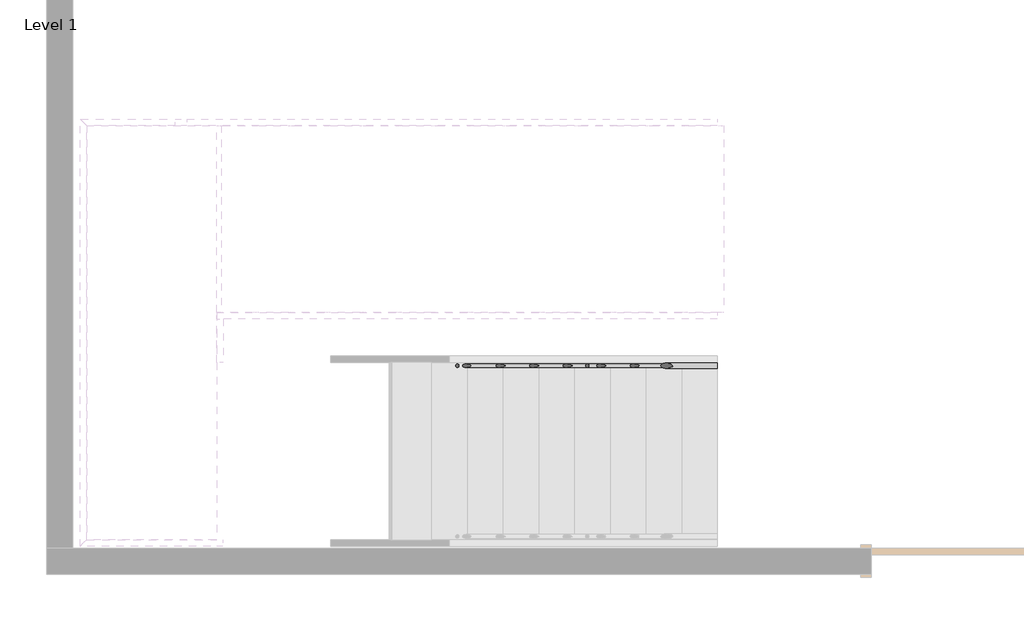
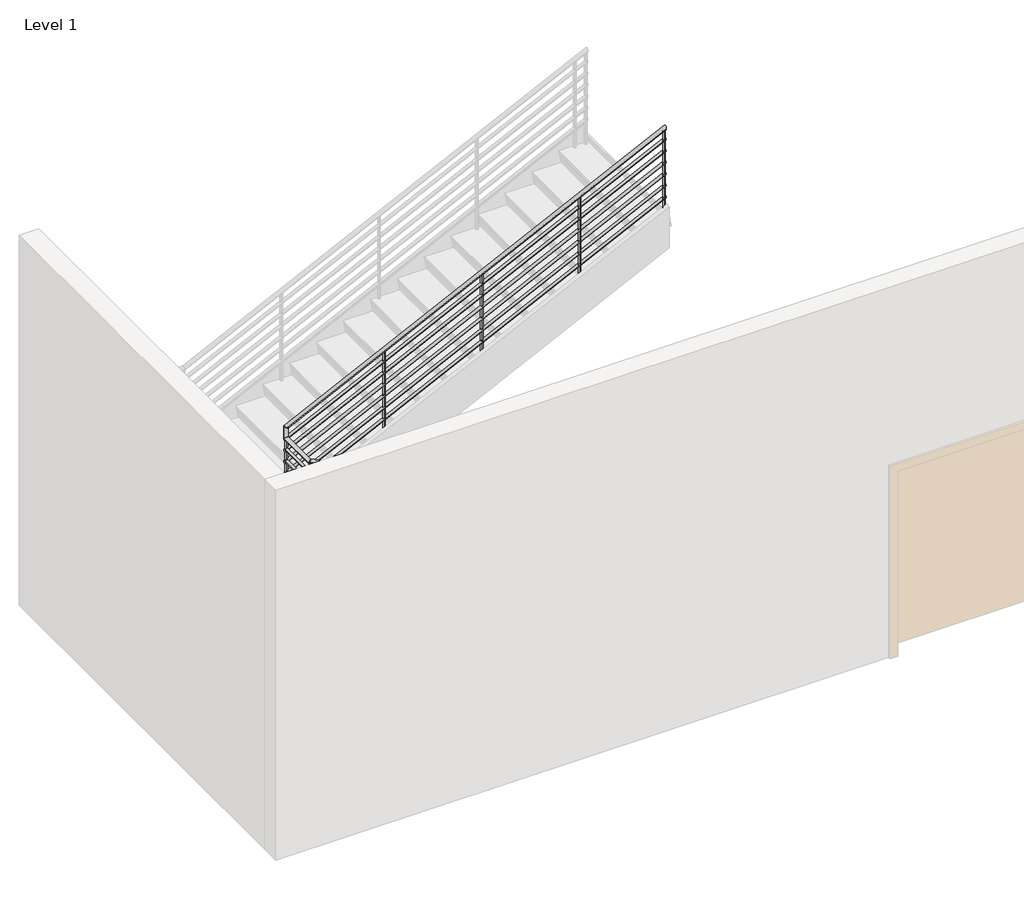
# One storey, part 2 of 4: 1 railing.
"""IFC4 building model written with IfcOpenShell, lengths in millimetres."""

from ifc_helpers import new_model, si_unit, point, frame, frame_2d, origin, place, context, project, spatial, circle_curve, ellipse_curve, trimmed, segment, composite_curve, outline, extrude, element, save
from ifc_brep_helpers import plane_surface, cylinder_surface, advanced_brep

model = new_model("IFC4")

# Units and contexts
model_context = context("Model", 3, world=origin())
ifc_project = project(units=[si_unit("LENGTHUNIT", "METRE", prefix="MILLI")], contexts=[model_context])

# Site, building, storey
site = spatial("IfcSite", under=ifc_project)
building = spatial("IfcBuilding", under=site)
storey = spatial("IfcBuildingStorey", under=building, Name="Level 1", Elevation=0.0)

# Railing
placement = place(None, origin())
element("IfcRailing", 1, ObjectType="900mm Pipe", at=placement, inside=storey, context=model_context, shape_type="SolidModel", body=[
    advanced_brep(
    [(3615.6033064, 209.9469597, 1011.1065202), (3615.6033064, 169.9469597, 1011.1065202), (-250.5258816, 209.9469597, 2885.5933992), (-286.5184459, 169.9469597, 2903.0443395)],
    [
        (0, 1, ellipse_curve(frame((3615.6033064, 189.9469597, 1011.1065202), z_axis=(1.0, 0.0, 0.0), x_axis=(0.0, 0.0, -1.0)), 22.2268131, 20.0)),
        (1, 0, ellipse_curve(frame((3615.6033064, 189.9469597, 1011.1065202), z_axis=(1.0, 0.0, 0.0), x_axis=(0.0, 0.0, -1.0)), 22.2268131, 20.0)),
        (2, 3, ellipse_curve(frame((-268.5221637, 189.9469597, 2894.3188694), z_axis=(-0.6362646570057477, 0.7071067811865508, 0.3084919549118802), x_axis=(0.6362646570057556, 0.7071067811865441, -0.30849195491187914)), 28.2842712, 20.0)),
        (3, 2, ellipse_curve(frame((-268.5221637, 189.9469597, 2894.3188694), z_axis=(-0.6362646570057477, 0.7071067811865508, 0.3084919549118802), x_axis=(0.6362646570057556, 0.7071067811865441, -0.30849195491187914)), 28.2842712, 20.0)),
        (0, 2),
        (3, 1),
    ],
    [
        plane_surface(frame((3615.6033064, 189.9469597, 1033.3333333), z_axis=(1.0, 0.0, 0.0), x_axis=(0.0, -1.0, 0.0))),
        plane_surface(frame((-259.7966936, 189.9469597, 2912.3151515), z_axis=(-0.6362646570057479, 0.7071067811865509, 0.30849195491188025), x_axis=(0.7714708589735313, 0.5831808789209693, 0.2544263669818984))),
        cylinder_surface(frame((3606.8778363, 189.9469597, 1015.3370512), z_axis=(0.8998141071961996, 0.0, -0.4362735065193696), x_axis=(0.0, -1.0, 0.0)), 20.0),
    ],
    [
        (0, [[1, 2]]),
        (1, [[3, 4]]),
        (2, [[-1, 5, -4, 6]]),
        (2, [[-2, -6, -3, -5]]),
    ],
),
    advanced_brep(
    [(-239.7966936, 216.668712, 2880.0), (-279.7966936, 180.6761477, 2880.0), (-239.7966936, 626.6300402, 2880.0), (-279.7966936, 626.6300402, 2880.0)],
    [
        (0, 1, ellipse_curve(frame((-259.7966936, 198.6724298, 2880.0), z_axis=(0.6362646570057477, -0.7071067811865508, -0.3084919549118802), x_axis=(-0.6362646570057556, -0.7071067811865442, 0.3084919549118791)), 28.2842712, 20.0)),
        (1, 0, ellipse_curve(frame((-259.7966936, 198.6724298, 2880.0), z_axis=(0.6362646570057477, -0.7071067811865508, -0.3084919549118802), x_axis=(-0.6362646570057556, -0.7071067811865442, 0.3084919549118791)), 28.2842712, 20.0)),
        (2, 3, ellipse_curve(frame((-259.7966936, 626.6300402, 2880.0), z_axis=(0.0, 0.7071067811865479, 0.7071067811865471), x_axis=(0.0, -0.7071067811865471, 0.7071067811865479)), 28.2842712, 20.0)),
        (3, 2, ellipse_curve(frame((-259.7966936, 626.6300402, 2880.0), z_axis=(0.0, 0.7071067811865479, 0.7071067811865471), x_axis=(0.0, -0.7071067811865471, 0.7071067811865479)), 28.2842712, 20.0)),
        (0, 2),
        (3, 1),
    ],
    [
        plane_surface(frame((-259.7966936, 189.9469597, 2900.0), z_axis=(0.6362646570057479, -0.7071067811865509, -0.30849195491188025), x_axis=(0.7714708589735313, 0.5831808789209693, 0.2544263669818984))),
        plane_surface(frame((-259.7966936, 606.6300402, 2900.0), z_axis=(0.0, 0.7071067811865479, 0.7071067811865471), x_axis=(1.0, 0.0, 0.0))),
        cylinder_surface(frame((-259.7966936, 189.9469597, 2880.0), z_axis=(0.0, -1.0, 0.0), x_axis=(-1.0, 0.0, 0.0)), 20.0),
    ],
    [
        (0, [[1, 2]]),
        (1, [[3, 4]]),
        (2, [[-1, 5, -4, 6]]),
        (2, [[-2, -6, -3, -5]]),
    ],
),
    advanced_brep(
    [(-239.7966936, 626.6300402, 2880.0), (-279.7966936, 626.6300402, 2880.0), (-239.7966936, 626.6300402, 2986.2615253), (-279.7966936, 626.6300402, 3011.3212121)],
    [
        (0, 1, ellipse_curve(frame((-259.7966936, 626.6300402, 2880.0), z_axis=(0.0, -0.7071067811865479, -0.7071067811865471), x_axis=(0.0, 0.7071067811865471, -0.7071067811865479)), 28.2842712, 20.0)),
        (1, 0, ellipse_curve(frame((-259.7966936, 626.6300402, 2880.0), z_axis=(0.0, -0.7071067811865479, -0.7071067811865471), x_axis=(0.0, 0.7071067811865471, -0.7071067811865479)), 28.2842712, 20.0)),
        (2, 3, ellipse_curve(frame((-259.7966936, 626.6300402, 2998.7913687), z_axis=(0.5309079456368263, 0.0, 0.8474294975156841), x_axis=(0.8474294975156841, 0.0, -0.530907945636826)), 23.6007834, 20.0)),
        (3, 2, ellipse_curve(frame((-259.7966936, 626.6300402, 2998.7913687), z_axis=(0.5309079456368263, 0.0, 0.8474294975156841), x_axis=(0.8474294975156841, 0.0, -0.530907945636826)), 23.6007834, 20.0)),
        (0, 2),
        (3, 1),
    ],
    [
        plane_surface(frame((-259.7966936, 626.6300402, 2880.0), z_axis=(0.0, -0.7071067811865479, -0.7071067811865471), x_axis=(1.0, 0.0, 0.0))),
        plane_surface(frame((-259.7966936, 626.6300402, 2998.7913687), z_axis=(0.5309079456368263, 0.0, 0.8474294975156841), x_axis=(0.8474294975156841, 0.0, -0.5309079456368263))),
        cylinder_surface(frame((-259.7966936, 626.6300402, 2880.0), z_axis=(0.0, 0.0, -1.0), x_axis=(-1.0, 0.0, 0.0)), 20.0),
    ],
    [
        (0, [[1, 2]]),
        (1, [[3, 4]]),
        (2, [[-1, 5, -4, 6]]),
        (2, [[-2, -6, -3, -5]]),
    ],
),
    advanced_brep(
    [(-259.7966936, 606.6300402, 2998.7913687), (-259.7966936, 646.6300402, 2998.7913687), (3615.6033064, 606.6300402, 4877.7731869), (3615.6033064, 646.6300402, 4877.7731869)],
    [
        (0, 1, ellipse_curve(frame((-259.7966936, 626.6300402, 2998.7913687), z_axis=(-0.5309079456368263, 0.0, -0.8474294975156841), x_axis=(-0.8474294975156837, 0.0, 0.5309079456368265)), 23.6007834, 20.0)),
        (1, 0, ellipse_curve(frame((-259.7966936, 626.6300402, 2998.7913687), z_axis=(-0.5309079456368263, 0.0, -0.8474294975156841), x_axis=(-0.8474294975156837, 0.0, 0.5309079456368265)), 23.6007834, 20.0)),
        (2, 3, ellipse_curve(frame((3615.6033064, 626.6300402, 4877.7731869), z_axis=(1.0, 0.0, 0.0), x_axis=(0.0, 0.0, -1.0)), 22.2268131, 20.0)),
        (3, 2, ellipse_curve(frame((3615.6033064, 626.6300402, 4877.7731869), z_axis=(1.0, 0.0, 0.0), x_axis=(0.0, 0.0, -1.0)), 22.2268131, 20.0)),
        (0, 2),
        (3, 1),
    ],
    [
        plane_surface(frame((-279.7966936, 626.6300402, 3011.3212121), z_axis=(-0.5309079456368263, 0.0, -0.8474294975156841), x_axis=(0.8474294975156841, 0.0, -0.5309079456368263))),
        plane_surface(frame((3615.6033064, 626.6300402, 4900.0), z_axis=(1.0, 0.0, 0.0), x_axis=(0.0, 1.0, 0.0))),
        cylinder_surface(frame((-271.0712235, 626.6300402, 2993.32493), z_axis=(-0.8998141071961995, 0.0, -0.4362735065193696), x_axis=(0.0, 1.0, 0.0)), 20.0),
    ],
    [
        (0, [[1, 2]]),
        (1, [[3, 4]]),
        (2, [[-1, 5, -4, 6]]),
        (2, [[-2, -6, -3, -5]]),
    ],
),
    advanced_brep(
    [(3615.6033064, 174.9469597, 891.6632235), (3615.6033064, 204.9469597, 891.6632235), (-237.8412951, 174.9469597, 2760.0), (-237.8412951, 204.9469597, 2760.0), (-274.7966936, 174.9469597, 2760.0), (-244.7966936, 204.9469597, 2760.0), (-274.7966936, 611.6300402, 2760.0), (-244.7966936, 611.6300402, 2760.0)],
    [
        (0, 1, ellipse_curve(frame((3615.6033064, 189.9469597, 891.6632235), z_axis=(1.0, 0.0, 0.0), x_axis=(0.0, 0.0, -1.0)), 16.6701098, 15.0)),
        (1, 0, ellipse_curve(frame((3615.6033064, 189.9469597, 891.6632235), z_axis=(1.0, 0.0, 0.0), x_axis=(0.0, 0.0, -1.0)), 16.6701098, 15.0)),
        (0, 2),
        (2, 3, ellipse_curve(frame((-237.8412951, 189.9469597, 2760.0), z_axis=(0.9746317528164674, 0.0, -0.22381453572522994), x_axis=(-0.2238145357252298, 0.0, -0.9746317528164675)), 15.3904282, 15.0)),
        (3, 1),
        (3, 2, ellipse_curve(frame((-237.8412951, 189.9469597, 2760.0), z_axis=(0.9746317528164674, 0.0, -0.22381453572522994), x_axis=(-0.2238145357252298, 0.0, -0.9746317528164675)), 15.3904282, 15.0)),
        (2, 4),
        (4, 5, ellipse_curve(frame((-259.7966936, 189.9469597, 2760.0), z_axis=(0.7071067811865438, -0.7071067811865513, 0.0), x_axis=(0.7071067811865511, 0.7071067811865439, 0.0)), 21.2132034, 15.0)),
        (5, 3),
        (5, 4, ellipse_curve(frame((-259.7966936, 189.9469597, 2760.0), z_axis=(0.7071067811865438, -0.7071067811865513, 0.0), x_axis=(0.7071067811865511, 0.7071067811865439, 0.0)), 21.2132034, 15.0)),
        (6, 7, circle_curve(frame((-259.7966936, 611.6300402, 2760.0), z_axis=(0.0, 1.0, 0.0), x_axis=(1.0, 0.0, 0.0)), 15.0)),
        (7, 6, circle_curve(frame((-259.7966936, 611.6300402, 2760.0), z_axis=(0.0, 1.0, 0.0), x_axis=(1.0, 0.0, 0.0)), 15.0)),
        (4, 6),
        (7, 5),
    ],
    [
        plane_surface(frame((3615.6033064, 189.9469597, 908.3333333), z_axis=(1.0, 0.0, 0.0), x_axis=(0.0, -1.0, 0.0))),
        cylinder_surface(frame((3609.0592038, 189.9469597, 894.8361217), z_axis=(0.8998141071961996, 0.0, -0.4362735065193695), x_axis=(0.0, 1.0, 0.0)), 15.0),
        cylinder_surface(frame((-234.3966936, 189.9469597, 2760.0), z_axis=(1.0, 0.0, 0.0), x_axis=(0.0, 1.0, 0.0)), 15.0),
        plane_surface(frame((-259.7966936, 611.6300402, 2775.0), z_axis=(0.0, 1.0, 0.0), x_axis=(0.0, 0.0, 1.0))),
        cylinder_surface(frame((-259.7966936, 189.9469597, 2760.0), z_axis=(0.0, -1.0, 0.0), x_axis=(1.0, 0.0, 0.0)), 15.0),
    ],
    [
        (0, [[1, 2]]),
        (1, [[-1, 3, 4, 5]]),
        (1, [[-2, -5, 6, -3]]),
        (2, [[-4, 7, 8, 9]]),
        (2, [[-6, -9, 10, -7]]),
        (3, [[11, 12]]),
        (4, [[-8, 13, -12, 14]]),
        (4, [[-10, -14, -11, -13]]),
    ],
),
    advanced_brep(
    [(-274.7966936, 641.6300402, 2872.0753447), (-274.7966936, 611.6300402, 2872.0753447), (3615.6033064, 641.6300402, 4758.3298902), (3615.6033064, 611.6300402, 4758.3298902)],
    [
        (0, 1, ellipse_curve(frame((-274.7966936, 626.6300402, 2872.0753447), z_axis=(-1.0, 0.0, 0.0), x_axis=(0.0, 0.0, -1.0)), 16.6701098, 15.0)),
        (1, 0, ellipse_curve(frame((-274.7966936, 626.6300402, 2872.0753447), z_axis=(-1.0, 0.0, 0.0), x_axis=(0.0, 0.0, -1.0)), 16.6701098, 15.0)),
        (2, 3, ellipse_curve(frame((3615.6033064, 626.6300402, 4758.3298902), z_axis=(1.0, 0.0, 0.0), x_axis=(0.0, 0.0, -1.0)), 16.6701098, 15.0)),
        (3, 2, ellipse_curve(frame((3615.6033064, 626.6300402, 4758.3298902), z_axis=(1.0, 0.0, 0.0), x_axis=(0.0, 0.0, -1.0)), 16.6701098, 15.0)),
        (0, 2),
        (3, 1),
    ],
    [
        plane_surface(frame((-274.7966936, 626.6300402, 2888.7454545), z_axis=(-1.0, 0.0, 0.0), x_axis=(0.0, 1.0, 0.0))),
        plane_surface(frame((3615.6033064, 626.6300402, 4775.0), z_axis=(1.0, 0.0, 0.0), x_axis=(0.0, 1.0, 0.0))),
        cylinder_surface(frame((-268.252591, 626.6300402, 2875.2482429), z_axis=(-0.8998141071961995, 0.0, -0.4362735065193696), x_axis=(0.0, -1.0, 0.0)), 15.0),
    ],
    [
        (0, [[1, 2]]),
        (1, [[3, 4]]),
        (2, [[-1, 5, -4, 6]]),
        (2, [[-2, -6, -3, -5]]),
    ],
),
    advanced_brep(
    [(3615.6033064, 174.9469597, 766.6632235), (3615.6033064, 204.9469597, 766.6632235), (-237.8412951, 174.9469597, 2635.0), (-237.8412951, 204.9469597, 2635.0), (-274.7966936, 174.9469597, 2635.0), (-244.7966936, 204.9469597, 2635.0), (-274.7966936, 611.6300402, 2635.0), (-244.7966936, 611.6300402, 2635.0)],
    [
        (0, 1, ellipse_curve(frame((3615.6033064, 189.9469597, 766.6632235), z_axis=(1.0, 0.0, 0.0), x_axis=(0.0, 0.0, -1.0)), 16.6701098, 15.0)),
        (1, 0, ellipse_curve(frame((3615.6033064, 189.9469597, 766.6632235), z_axis=(1.0, 0.0, 0.0), x_axis=(0.0, 0.0, -1.0)), 16.6701098, 15.0)),
        (0, 2),
        (2, 3, ellipse_curve(frame((-237.8412951, 189.9469597, 2635.0), z_axis=(0.9746317528164674, 0.0, -0.22381453572522994), x_axis=(-0.2238145357252298, 0.0, -0.9746317528164675)), 15.3904282, 15.0)),
        (3, 1),
        (3, 2, ellipse_curve(frame((-237.8412951, 189.9469597, 2635.0), z_axis=(0.9746317528164674, 0.0, -0.22381453572522994), x_axis=(-0.2238145357252298, 0.0, -0.9746317528164675)), 15.3904282, 15.0)),
        (2, 4),
        (4, 5, ellipse_curve(frame((-259.7966936, 189.9469597, 2635.0), z_axis=(0.7071067811865438, -0.7071067811865513, 0.0), x_axis=(0.7071067811865511, 0.7071067811865439, 0.0)), 21.2132034, 15.0)),
        (5, 3),
        (5, 4, ellipse_curve(frame((-259.7966936, 189.9469597, 2635.0), z_axis=(0.7071067811865438, -0.7071067811865513, 0.0), x_axis=(0.7071067811865511, 0.7071067811865439, 0.0)), 21.2132034, 15.0)),
        (6, 7, circle_curve(frame((-259.7966936, 611.6300402, 2635.0), z_axis=(0.0, 1.0, 0.0), x_axis=(1.0, 0.0, 0.0)), 15.0)),
        (7, 6, circle_curve(frame((-259.7966936, 611.6300402, 2635.0), z_axis=(0.0, 1.0, 0.0), x_axis=(1.0, 0.0, 0.0)), 15.0)),
        (4, 6),
        (7, 5),
    ],
    [
        plane_surface(frame((3615.6033064, 189.9469597, 783.3333333), z_axis=(1.0, 0.0, 0.0), x_axis=(0.0, -1.0, 0.0))),
        cylinder_surface(frame((3609.0592038, 189.9469597, 769.8361217), z_axis=(0.8998141071961996, 0.0, -0.4362735065193695), x_axis=(0.0, 1.0, 0.0)), 15.0),
        cylinder_surface(frame((-234.3966936, 189.9469597, 2635.0), z_axis=(1.0, 0.0, 0.0), x_axis=(0.0, 1.0, 0.0)), 15.0),
        plane_surface(frame((-259.7966936, 611.6300402, 2650.0), z_axis=(0.0, 1.0, 0.0), x_axis=(0.0, 0.0, 1.0))),
        cylinder_surface(frame((-259.7966936, 189.9469597, 2635.0), z_axis=(0.0, -1.0, 0.0), x_axis=(1.0, 0.0, 0.0)), 15.0),
    ],
    [
        (0, [[1, 2]]),
        (1, [[-1, 3, 4, 5]]),
        (1, [[-2, -5, 6, -3]]),
        (2, [[-4, 7, 8, 9]]),
        (2, [[-6, -9, 10, -7]]),
        (3, [[11, 12]]),
        (4, [[-8, 13, -12, 14]]),
        (4, [[-10, -14, -11, -13]]),
    ],
),
    advanced_brep(
    [(-274.7966936, 641.6300402, 2747.0753447), (-274.7966936, 611.6300402, 2747.0753447), (3615.6033064, 641.6300402, 4633.3298902), (3615.6033064, 611.6300402, 4633.3298902)],
    [
        (0, 1, ellipse_curve(frame((-274.7966936, 626.6300402, 2747.0753447), z_axis=(-1.0, 0.0, 0.0), x_axis=(0.0, 0.0, -1.0)), 16.6701098, 15.0)),
        (1, 0, ellipse_curve(frame((-274.7966936, 626.6300402, 2747.0753447), z_axis=(-1.0, 0.0, 0.0), x_axis=(0.0, 0.0, -1.0)), 16.6701098, 15.0)),
        (2, 3, ellipse_curve(frame((3615.6033064, 626.6300402, 4633.3298902), z_axis=(1.0, 0.0, 0.0), x_axis=(0.0, 0.0, -1.0)), 16.6701098, 15.0)),
        (3, 2, ellipse_curve(frame((3615.6033064, 626.6300402, 4633.3298902), z_axis=(1.0, 0.0, 0.0), x_axis=(0.0, 0.0, -1.0)), 16.6701098, 15.0)),
        (0, 2),
        (3, 1),
    ],
    [
        plane_surface(frame((-274.7966936, 626.6300402, 2763.7454545), z_axis=(-1.0, 0.0, 0.0), x_axis=(0.0, 1.0, 0.0))),
        plane_surface(frame((3615.6033064, 626.6300402, 4650.0), z_axis=(1.0, 0.0, 0.0), x_axis=(0.0, 1.0, 0.0))),
        cylinder_surface(frame((-268.252591, 626.6300402, 2750.2482429), z_axis=(-0.8998141071961996, 0.0, -0.4362735065193695), x_axis=(0.0, -1.0, 0.0)), 15.0),
    ],
    [
        (0, [[1, 2]]),
        (1, [[3, 4]]),
        (2, [[-1, 5, -4, 6]]),
        (2, [[-2, -6, -3, -5]]),
    ],
),
    advanced_brep(
    [(3615.6033064, 174.9469597, 641.6632235), (3615.6033064, 204.9469597, 641.6632235), (-237.8412951, 174.9469597, 2510.0), (-237.8412951, 204.9469597, 2510.0), (-274.7966936, 174.9469597, 2510.0), (-244.7966936, 204.9469597, 2510.0), (-274.7966936, 611.6300402, 2510.0), (-244.7966936, 611.6300402, 2510.0)],
    [
        (0, 1, ellipse_curve(frame((3615.6033064, 189.9469597, 641.6632235), z_axis=(1.0, 0.0, 0.0), x_axis=(0.0, 0.0, -1.0)), 16.6701098, 15.0)),
        (1, 0, ellipse_curve(frame((3615.6033064, 189.9469597, 641.6632235), z_axis=(1.0, 0.0, 0.0), x_axis=(0.0, 0.0, -1.0)), 16.6701098, 15.0)),
        (0, 2),
        (2, 3, ellipse_curve(frame((-237.8412951, 189.9469597, 2510.0), z_axis=(0.9746317528164674, 0.0, -0.2238145357252299), x_axis=(-0.22381453572522944, 0.0, -0.9746317528164676)), 15.3904282, 15.0)),
        (3, 1),
        (3, 2, ellipse_curve(frame((-237.8412951, 189.9469597, 2510.0), z_axis=(0.9746317528164674, 0.0, -0.2238145357252299), x_axis=(-0.22381453572522944, 0.0, -0.9746317528164676)), 15.3904282, 15.0)),
        (2, 4),
        (4, 5, ellipse_curve(frame((-259.7966936, 189.9469597, 2510.0), z_axis=(0.7071067811865438, -0.7071067811865513, 0.0), x_axis=(0.7071067811865511, 0.7071067811865439, 0.0)), 21.2132034, 15.0)),
        (5, 3),
        (5, 4, ellipse_curve(frame((-259.7966936, 189.9469597, 2510.0), z_axis=(0.7071067811865438, -0.7071067811865513, 0.0), x_axis=(0.7071067811865511, 0.7071067811865439, 0.0)), 21.2132034, 15.0)),
        (6, 7, circle_curve(frame((-259.7966936, 611.6300402, 2510.0), z_axis=(0.0, 1.0, 0.0), x_axis=(1.0, 0.0, 0.0)), 15.0)),
        (7, 6, circle_curve(frame((-259.7966936, 611.6300402, 2510.0), z_axis=(0.0, 1.0, 0.0), x_axis=(1.0, 0.0, 0.0)), 15.0)),
        (4, 6),
        (7, 5),
    ],
    [
        plane_surface(frame((3615.6033064, 189.9469597, 658.3333333), z_axis=(1.0, 0.0, 0.0), x_axis=(0.0, -1.0, 0.0))),
        cylinder_surface(frame((3609.0592038, 189.9469597, 644.8361217), z_axis=(0.8998141071961997, 0.0, -0.4362735065193694), x_axis=(0.0, 1.0, 0.0)), 15.0),
        cylinder_surface(frame((-234.3966936, 189.9469597, 2510.0), z_axis=(1.0, 0.0, 0.0), x_axis=(0.0, 1.0, 0.0)), 15.0),
        plane_surface(frame((-259.7966936, 611.6300402, 2525.0), z_axis=(0.0, 1.0, 0.0), x_axis=(0.0, 0.0, 1.0))),
        cylinder_surface(frame((-259.7966936, 189.9469597, 2510.0), z_axis=(0.0, -1.0, 0.0), x_axis=(1.0, 0.0, 0.0)), 15.0),
    ],
    [
        (0, [[1, 2]]),
        (1, [[-1, 3, 4, 5]]),
        (1, [[-2, -5, 6, -3]]),
        (2, [[-4, 7, 8, 9]]),
        (2, [[-6, -9, 10, -7]]),
        (3, [[11, 12]]),
        (4, [[-8, 13, -12, 14]]),
        (4, [[-10, -14, -11, -13]]),
    ],
),
    advanced_brep(
    [(-274.7966936, 641.6300402, 2622.0753447), (-274.7966936, 611.6300402, 2622.0753447), (3615.6033064, 641.6300402, 4508.3298902), (3615.6033064, 611.6300402, 4508.3298902)],
    [
        (0, 1, ellipse_curve(frame((-274.7966936, 626.6300402, 2622.0753447), z_axis=(-1.0, 0.0, 0.0), x_axis=(0.0, 0.0, -1.0)), 16.6701098, 15.0)),
        (1, 0, ellipse_curve(frame((-274.7966936, 626.6300402, 2622.0753447), z_axis=(-1.0, 0.0, 0.0), x_axis=(0.0, 0.0, -1.0)), 16.6701098, 15.0)),
        (2, 3, ellipse_curve(frame((3615.6033064, 626.6300402, 4508.3298902), z_axis=(1.0, 0.0, 0.0), x_axis=(0.0, 0.0, -1.0)), 16.6701098, 15.0)),
        (3, 2, ellipse_curve(frame((3615.6033064, 626.6300402, 4508.3298902), z_axis=(1.0, 0.0, 0.0), x_axis=(0.0, 0.0, -1.0)), 16.6701098, 15.0)),
        (0, 2),
        (3, 1),
    ],
    [
        plane_surface(frame((-274.7966936, 626.6300402, 2638.7454545), z_axis=(-1.0, 0.0, 0.0), x_axis=(0.0, 1.0, 0.0))),
        plane_surface(frame((3615.6033064, 626.6300402, 4525.0), z_axis=(1.0, 0.0, 0.0), x_axis=(0.0, 1.0, 0.0))),
        cylinder_surface(frame((-268.252591, 626.6300402, 2625.2482429), z_axis=(-0.8998141071961996, 0.0, -0.4362735065193695), x_axis=(0.0, -1.0, 0.0)), 15.0),
    ],
    [
        (0, [[1, 2]]),
        (1, [[3, 4]]),
        (2, [[-1, 5, -4, 6]]),
        (2, [[-2, -6, -3, -5]]),
    ],
),
    advanced_brep(
    [(3615.6033064, 174.9469597, 516.6632235), (3615.6033064, 204.9469597, 516.6632235), (-237.8412951, 174.9469597, 2385.0), (-237.8412951, 204.9469597, 2385.0), (-274.7966936, 174.9469597, 2385.0), (-244.7966936, 204.9469597, 2385.0), (-274.7966936, 611.6300402, 2385.0), (-244.7966936, 611.6300402, 2385.0)],
    [
        (0, 1, ellipse_curve(frame((3615.6033064, 189.9469597, 516.6632235), z_axis=(1.0, 0.0, 0.0), x_axis=(0.0, 0.0, -1.0)), 16.6701098, 15.0)),
        (1, 0, ellipse_curve(frame((3615.6033064, 189.9469597, 516.6632235), z_axis=(1.0, 0.0, 0.0), x_axis=(0.0, 0.0, -1.0)), 16.6701098, 15.0)),
        (0, 2),
        (2, 3, ellipse_curve(frame((-237.8412951, 189.9469597, 2385.0), z_axis=(0.9746317528164674, 0.0, -0.22381453572522994), x_axis=(-0.2238145357252298, 0.0, -0.9746317528164675)), 15.3904282, 15.0)),
        (3, 1),
        (3, 2, ellipse_curve(frame((-237.8412951, 189.9469597, 2385.0), z_axis=(0.9746317528164674, 0.0, -0.22381453572522994), x_axis=(-0.2238145357252298, 0.0, -0.9746317528164675)), 15.3904282, 15.0)),
        (2, 4),
        (4, 5, ellipse_curve(frame((-259.7966936, 189.9469597, 2385.0), z_axis=(0.7071067811865438, -0.7071067811865513, 0.0), x_axis=(0.7071067811865511, 0.7071067811865439, 0.0)), 21.2132034, 15.0)),
        (5, 3),
        (5, 4, ellipse_curve(frame((-259.7966936, 189.9469597, 2385.0), z_axis=(0.7071067811865438, -0.7071067811865513, 0.0), x_axis=(0.7071067811865511, 0.7071067811865439, 0.0)), 21.2132034, 15.0)),
        (6, 7, circle_curve(frame((-259.7966936, 611.6300402, 2385.0), z_axis=(0.0, 1.0, 0.0), x_axis=(1.0, 0.0, 0.0)), 15.0)),
        (7, 6, circle_curve(frame((-259.7966936, 611.6300402, 2385.0), z_axis=(0.0, 1.0, 0.0), x_axis=(1.0, 0.0, 0.0)), 15.0)),
        (4, 6),
        (7, 5),
    ],
    [
        plane_surface(frame((3615.6033064, 189.9469597, 533.3333333), z_axis=(1.0, 0.0, 0.0), x_axis=(0.0, -1.0, 0.0))),
        cylinder_surface(frame((3609.0592038, 189.9469597, 519.8361217), z_axis=(0.8998141071961996, 0.0, -0.4362735065193695), x_axis=(0.0, 1.0, 0.0)), 15.0),
        cylinder_surface(frame((-234.3966936, 189.9469597, 2385.0), z_axis=(1.0, 0.0, 0.0), x_axis=(0.0, 1.0, 0.0)), 15.0),
        plane_surface(frame((-259.7966936, 611.6300402, 2400.0), z_axis=(0.0, 1.0, 0.0), x_axis=(0.0, 0.0, 1.0))),
        cylinder_surface(frame((-259.7966936, 189.9469597, 2385.0), z_axis=(0.0, -1.0, 0.0), x_axis=(1.0, 0.0, 0.0)), 15.0),
    ],
    [
        (0, [[1, 2]]),
        (1, [[-1, 3, 4, 5]]),
        (1, [[-2, -5, 6, -3]]),
        (2, [[-4, 7, 8, 9]]),
        (2, [[-6, -9, 10, -7]]),
        (3, [[11, 12]]),
        (4, [[-8, 13, -12, 14]]),
        (4, [[-10, -14, -11, -13]]),
    ],
),
    advanced_brep(
    [(-274.7966936, 641.6300402, 2497.0753447), (-274.7966936, 611.6300402, 2497.0753447), (3615.6033064, 641.6300402, 4383.3298902), (3615.6033064, 611.6300402, 4383.3298902)],
    [
        (0, 1, ellipse_curve(frame((-274.7966936, 626.6300402, 2497.0753447), z_axis=(-1.0, 0.0, 0.0), x_axis=(0.0, 0.0, -1.0)), 16.6701098, 15.0)),
        (1, 0, ellipse_curve(frame((-274.7966936, 626.6300402, 2497.0753447), z_axis=(-1.0, 0.0, 0.0), x_axis=(0.0, 0.0, -1.0)), 16.6701098, 15.0)),
        (2, 3, ellipse_curve(frame((3615.6033064, 626.6300402, 4383.3298902), z_axis=(1.0, 0.0, 0.0), x_axis=(0.0, 0.0, -1.0)), 16.6701098, 15.0)),
        (3, 2, ellipse_curve(frame((3615.6033064, 626.6300402, 4383.3298902), z_axis=(1.0, 0.0, 0.0), x_axis=(0.0, 0.0, -1.0)), 16.6701098, 15.0)),
        (0, 2),
        (3, 1),
    ],
    [
        plane_surface(frame((-274.7966936, 626.6300402, 2513.7454545), z_axis=(-1.0, 0.0, 0.0), x_axis=(0.0, 1.0, 0.0))),
        plane_surface(frame((3615.6033064, 626.6300402, 4400.0), z_axis=(1.0, 0.0, 0.0), x_axis=(0.0, 1.0, 0.0))),
        cylinder_surface(frame((-268.252591, 626.6300402, 2500.2482429), z_axis=(-0.8998141071961995, 0.0, -0.4362735065193696), x_axis=(0.0, -1.0, 0.0)), 15.0),
    ],
    [
        (0, [[1, 2]]),
        (1, [[3, 4]]),
        (2, [[-1, 5, -4, 6]]),
        (2, [[-2, -6, -3, -5]]),
    ],
),
    advanced_brep(
    [(3615.6033064, 174.9469597, 391.6632235), (3615.6033064, 204.9469597, 391.6632235), (-237.8412951, 174.9469597, 2260.0), (-237.8412951, 204.9469597, 2260.0), (-274.7966936, 174.9469597, 2260.0), (-244.7966936, 204.9469597, 2260.0), (-274.7966936, 611.6300402, 2260.0), (-244.7966936, 611.6300402, 2260.0)],
    [
        (0, 1, ellipse_curve(frame((3615.6033064, 189.9469597, 391.6632235), z_axis=(1.0, 0.0, 0.0), x_axis=(0.0, 0.0, -1.0)), 16.6701098, 15.0)),
        (1, 0, ellipse_curve(frame((3615.6033064, 189.9469597, 391.6632235), z_axis=(1.0, 0.0, 0.0), x_axis=(0.0, 0.0, -1.0)), 16.6701098, 15.0)),
        (0, 2),
        (2, 3, ellipse_curve(frame((-237.8412951, 189.9469597, 2260.0), z_axis=(0.9746317528164674, 0.0, -0.22381453572522994), x_axis=(-0.2238145357252298, 0.0, -0.9746317528164675)), 15.3904282, 15.0)),
        (3, 1),
        (3, 2, ellipse_curve(frame((-237.8412951, 189.9469597, 2260.0), z_axis=(0.9746317528164674, 0.0, -0.22381453572522994), x_axis=(-0.2238145357252298, 0.0, -0.9746317528164675)), 15.3904282, 15.0)),
        (2, 4),
        (4, 5, ellipse_curve(frame((-259.7966936, 189.9469597, 2260.0), z_axis=(0.7071067811865438, -0.7071067811865513, 0.0), x_axis=(0.7071067811865511, 0.7071067811865439, 0.0)), 21.2132034, 15.0)),
        (5, 3),
        (5, 4, ellipse_curve(frame((-259.7966936, 189.9469597, 2260.0), z_axis=(0.7071067811865438, -0.7071067811865513, 0.0), x_axis=(0.7071067811865511, 0.7071067811865439, 0.0)), 21.2132034, 15.0)),
        (6, 7, circle_curve(frame((-259.7966936, 611.6300402, 2260.0), z_axis=(0.0, 1.0, 0.0), x_axis=(1.0, 0.0, 0.0)), 15.0)),
        (7, 6, circle_curve(frame((-259.7966936, 611.6300402, 2260.0), z_axis=(0.0, 1.0, 0.0), x_axis=(1.0, 0.0, 0.0)), 15.0)),
        (4, 6),
        (7, 5),
    ],
    [
        plane_surface(frame((3615.6033064, 189.9469597, 408.3333333), z_axis=(1.0, 0.0, 0.0), x_axis=(0.0, -1.0, 0.0))),
        cylinder_surface(frame((3609.0592038, 189.9469597, 394.8361217), z_axis=(0.8998141071961996, 0.0, -0.4362735065193695), x_axis=(0.0, 1.0, 0.0)), 15.0),
        cylinder_surface(frame((-234.3966936, 189.9469597, 2260.0), z_axis=(1.0, 0.0, 0.0), x_axis=(0.0, 1.0, 0.0)), 15.0),
        plane_surface(frame((-259.7966936, 611.6300402, 2275.0), z_axis=(0.0, 1.0, 0.0), x_axis=(0.0, 0.0, 1.0))),
        cylinder_surface(frame((-259.7966936, 189.9469597, 2260.0), z_axis=(0.0, -1.0, 0.0), x_axis=(1.0, 0.0, 0.0)), 15.0),
    ],
    [
        (0, [[1, 2]]),
        (1, [[-1, 3, 4, 5]]),
        (1, [[-2, -5, 6, -3]]),
        (2, [[-4, 7, 8, 9]]),
        (2, [[-6, -9, 10, -7]]),
        (3, [[11, 12]]),
        (4, [[-8, 13, -12, 14]]),
        (4, [[-10, -14, -11, -13]]),
    ],
),
    advanced_brep(
    [(-274.7966936, 641.6300402, 2372.0753447), (-274.7966936, 611.6300402, 2372.0753447), (3615.6033064, 641.6300402, 4258.3298902), (3615.6033064, 611.6300402, 4258.3298902)],
    [
        (0, 1, ellipse_curve(frame((-274.7966936, 626.6300402, 2372.0753447), z_axis=(-1.0, 0.0, 0.0), x_axis=(0.0, 0.0, -1.0)), 16.6701098, 15.0)),
        (1, 0, ellipse_curve(frame((-274.7966936, 626.6300402, 2372.0753447), z_axis=(-1.0, 0.0, 0.0), x_axis=(0.0, 0.0, -1.0)), 16.6701098, 15.0)),
        (2, 3, ellipse_curve(frame((3615.6033064, 626.6300402, 4258.3298902), z_axis=(1.0, 0.0, 0.0), x_axis=(0.0, 0.0, -1.0)), 16.6701098, 15.0)),
        (3, 2, ellipse_curve(frame((3615.6033064, 626.6300402, 4258.3298902), z_axis=(1.0, 0.0, 0.0), x_axis=(0.0, 0.0, -1.0)), 16.6701098, 15.0)),
        (0, 2),
        (3, 1),
    ],
    [
        plane_surface(frame((-274.7966936, 626.6300402, 2388.7454545), z_axis=(-1.0, 0.0, 0.0), x_axis=(0.0, 1.0, 0.0))),
        plane_surface(frame((3615.6033064, 626.6300402, 4275.0), z_axis=(1.0, 0.0, 0.0), x_axis=(0.0, 1.0, 0.0))),
        cylinder_surface(frame((-268.252591, 626.6300402, 2375.2482429), z_axis=(-0.8998141071961995, 0.0, -0.4362735065193696), x_axis=(0.0, -1.0, 0.0)), 15.0),
    ],
    [
        (0, [[1, 2]]),
        (1, [[3, 4]]),
        (2, [[-1, 5, -4, 6]]),
        (2, [[-2, -6, -3, -5]]),
    ],
),
    advanced_brep(
    [(3615.6033064, 174.9469597, 266.6632235), (3615.6033064, 204.9469597, 266.6632235), (-237.8412951, 174.9469597, 2135.0), (-237.8412951, 204.9469597, 2135.0), (-274.7966936, 174.9469597, 2135.0), (-244.7966936, 204.9469597, 2135.0), (-274.7966936, 611.6300402, 2135.0), (-244.7966936, 611.6300402, 2135.0)],
    [
        (0, 1, ellipse_curve(frame((3615.6033064, 189.9469597, 266.6632235), z_axis=(1.0, 0.0, 0.0), x_axis=(0.0, 0.0, -1.0)), 16.6701098, 15.0)),
        (1, 0, ellipse_curve(frame((3615.6033064, 189.9469597, 266.6632235), z_axis=(1.0, 0.0, 0.0), x_axis=(0.0, 0.0, -1.0)), 16.6701098, 15.0)),
        (0, 2),
        (2, 3, ellipse_curve(frame((-237.8412951, 189.9469597, 2135.0), z_axis=(0.9746317528164674, 0.0, -0.22381453572522994), x_axis=(-0.2238145357252298, 0.0, -0.9746317528164675)), 15.3904282, 15.0)),
        (3, 1),
        (3, 2, ellipse_curve(frame((-237.8412951, 189.9469597, 2135.0), z_axis=(0.9746317528164674, 0.0, -0.22381453572522994), x_axis=(-0.2238145357252298, 0.0, -0.9746317528164675)), 15.3904282, 15.0)),
        (2, 4),
        (4, 5, ellipse_curve(frame((-259.7966936, 189.9469597, 2135.0), z_axis=(0.7071067811865438, -0.7071067811865513, 0.0), x_axis=(0.7071067811865511, 0.7071067811865439, 0.0)), 21.2132034, 15.0)),
        (5, 3),
        (5, 4, ellipse_curve(frame((-259.7966936, 189.9469597, 2135.0), z_axis=(0.7071067811865438, -0.7071067811865513, 0.0), x_axis=(0.7071067811865511, 0.7071067811865439, 0.0)), 21.2132034, 15.0)),
        (6, 7, circle_curve(frame((-259.7966936, 611.6300402, 2135.0), z_axis=(0.0, 1.0, 0.0), x_axis=(1.0, 0.0, 0.0)), 15.0)),
        (7, 6, circle_curve(frame((-259.7966936, 611.6300402, 2135.0), z_axis=(0.0, 1.0, 0.0), x_axis=(1.0, 0.0, 0.0)), 15.0)),
        (4, 6),
        (7, 5),
    ],
    [
        plane_surface(frame((3615.6033064, 189.9469597, 283.3333333), z_axis=(1.0, 0.0, 0.0), x_axis=(0.0, -1.0, 0.0))),
        cylinder_surface(frame((3609.0592038, 189.9469597, 269.8361217), z_axis=(0.8998141071961996, 0.0, -0.4362735065193695), x_axis=(0.0, 1.0, 0.0)), 15.0),
        cylinder_surface(frame((-234.3966936, 189.9469597, 2135.0), z_axis=(1.0, 0.0, 0.0), x_axis=(0.0, 1.0, 0.0)), 15.0),
        plane_surface(frame((-259.7966936, 611.6300402, 2150.0), z_axis=(0.0, 1.0, 0.0), x_axis=(0.0, 0.0, 1.0))),
        cylinder_surface(frame((-259.7966936, 189.9469597, 2135.0), z_axis=(0.0, -1.0, 0.0), x_axis=(1.0, 0.0, 0.0)), 15.0),
    ],
    [
        (0, [[1, 2]]),
        (1, [[-1, 3, 4, 5]]),
        (1, [[-2, -5, 6, -3]]),
        (2, [[-4, 7, 8, 9]]),
        (2, [[-6, -9, 10, -7]]),
        (3, [[11, 12]]),
        (4, [[-8, 13, -12, 14]]),
        (4, [[-10, -14, -11, -13]]),
    ],
),
    advanced_brep(
    [(-274.7966936, 641.6300402, 2247.0753447), (-274.7966936, 611.6300402, 2247.0753447), (3615.6033064, 641.6300402, 4133.3298902), (3615.6033064, 611.6300402, 4133.3298902)],
    [
        (0, 1, ellipse_curve(frame((-274.7966936, 626.6300402, 2247.0753447), z_axis=(-1.0, 0.0, 0.0), x_axis=(0.0, 0.0, -1.0)), 16.6701098, 15.0)),
        (1, 0, ellipse_curve(frame((-274.7966936, 626.6300402, 2247.0753447), z_axis=(-1.0, 0.0, 0.0), x_axis=(0.0, 0.0, -1.0)), 16.6701098, 15.0)),
        (2, 3, ellipse_curve(frame((3615.6033064, 626.6300402, 4133.3298902), z_axis=(1.0, 0.0, 0.0), x_axis=(0.0, 0.0, -1.0)), 16.6701098, 15.0)),
        (3, 2, ellipse_curve(frame((3615.6033064, 626.6300402, 4133.3298902), z_axis=(1.0, 0.0, 0.0), x_axis=(0.0, 0.0, -1.0)), 16.6701098, 15.0)),
        (0, 2),
        (3, 1),
    ],
    [
        plane_surface(frame((-274.7966936, 626.6300402, 2263.7454545), z_axis=(-1.0, 0.0, 0.0), x_axis=(0.0, 1.0, 0.0))),
        plane_surface(frame((3615.6033064, 626.6300402, 4150.0), z_axis=(1.0, 0.0, 0.0), x_axis=(0.0, 1.0, 0.0))),
        cylinder_surface(frame((-268.252591, 626.6300402, 2250.2482429), z_axis=(-0.8998141071961995, 0.0, -0.4362735065193695), x_axis=(0.0, -1.0, 0.0)), 15.0),
    ],
    [
        (0, [[1, 2]]),
        (1, [[3, 4]]),
        (2, [[-1, 5, -4, 6]]),
        (2, [[-2, -6, -3, -5]]),
    ],
),
    advanced_brep(
    [(2740.2033064, 614.1300402, 4431.1100101), (2740.2033064, 614.1300402, 3466.6666667), (2740.2033064, 639.1300402, 3466.6666667), (2740.2033064, 639.1300402, 4431.1100101)],
    [
        (0, 1),
        (1, 2, circle_curve(frame((2740.2033064, 626.6300402, 3466.6666667), z_axis=(0.0, 0.0, 1.0), x_axis=(0.0, 1.0, 0.0)), 12.5)),
        (2, 3),
        (3, 0, ellipse_curve(frame((2740.2033064, 626.6300402, 4431.1100101), z_axis=(0.4362735065193688, 0.0, -0.8998141071961999), x_axis=(0.8998141071961999, 0.0, 0.4362735065193686)), 13.8917582, 12.5)),
        (0, 3, ellipse_curve(frame((2740.2033064, 626.6300402, 4431.1100101), z_axis=(0.4362735065193688, 0.0, -0.8998141071961999), x_axis=(0.8998141071961999, 0.0, 0.4362735065193686)), 13.8917582, 12.5)),
        (2, 1, circle_curve(frame((2740.2033064, 626.6300402, 3466.6666667), z_axis=(0.0, 0.0, 1.0), x_axis=(0.0, 1.0, 0.0)), 12.5)),
    ],
    [
        cylinder_surface(frame((2740.2033064, 626.6300402, 3366.6666667), z_axis=(0.0, 0.0, 1.0), x_axis=(0.0, 1.0, 0.0)), 12.5),
        plane_surface(frame((2765.2033064, 651.6300402, 4443.2312223), z_axis=(-0.4362735065193688, 0.0, 0.8998141071961999), x_axis=(0.0, -1.0, 0.0))),
        plane_surface(frame((2715.2033064, 651.6300402, 3466.6666667), z_axis=(0.0, 0.0, -1.0), x_axis=(0.0, -1.0, 0.0))),
    ],
    [
        (0, [[1, 2, 3, 4]]),
        (0, [[-1, 5, -3, 6]]),
        (1, [[-4, -5]]),
        (2, [[-2, -6]]),
    ],
),
    advanced_brep(
    [(1740.2033064, 614.1300402, 3946.2615253), (1740.2033064, 614.1300402, 3066.6666667), (1740.2033064, 639.1300402, 3066.6666667), (1740.2033064, 639.1300402, 3946.2615253)],
    [
        (0, 1),
        (1, 2, circle_curve(frame((1740.2033064, 626.6300402, 3066.6666667), z_axis=(0.0, 0.0, 1.0), x_axis=(0.0, 1.0, 0.0)), 12.5)),
        (2, 3),
        (3, 0, ellipse_curve(frame((1740.2033064, 626.6300402, 3946.2615253), z_axis=(0.4362735065193688, 0.0, -0.8998141071961999), x_axis=(0.8998141071961999, 0.0, 0.4362735065193686)), 13.8917582, 12.5)),
        (0, 3, ellipse_curve(frame((1740.2033064, 626.6300402, 3946.2615253), z_axis=(0.4362735065193688, 0.0, -0.8998141071961999), x_axis=(0.8998141071961999, 0.0, 0.4362735065193686)), 13.8917582, 12.5)),
        (2, 1, circle_curve(frame((1740.2033064, 626.6300402, 3066.6666667), z_axis=(0.0, 0.0, 1.0), x_axis=(0.0, 1.0, 0.0)), 12.5)),
    ],
    [
        cylinder_surface(frame((1740.2033064, 626.6300402, 2966.6666667), z_axis=(0.0, 0.0, 1.0), x_axis=(0.0, 1.0, 0.0)), 12.5),
        plane_surface(frame((1765.2033064, 651.6300402, 3958.3827374), z_axis=(-0.4362735065193688, 0.0, 0.8998141071961999), x_axis=(0.0, -1.0, 0.0))),
        plane_surface(frame((1715.2033064, 651.6300402, 3066.6666667), z_axis=(0.0, 0.0, -1.0), x_axis=(0.0, -1.0, 0.0))),
    ],
    [
        (0, [[1, 2, 3, 4]]),
        (0, [[-1, 5, -3, 6]]),
        (1, [[-4, -5]]),
        (2, [[-2, -6]]),
    ],
),
    advanced_brep(
    [(740.2033064, 614.1300402, 3461.4130404), (740.2033064, 614.1300402, 2533.3333333), (740.2033064, 639.1300402, 2533.3333333), (740.2033064, 639.1300402, 3461.4130404)],
    [
        (0, 1),
        (1, 2, circle_curve(frame((740.2033064, 626.6300402, 2533.3333333), z_axis=(0.0, 0.0, 1.0), x_axis=(0.0, 1.0, 0.0)), 12.5)),
        (2, 3),
        (3, 0, ellipse_curve(frame((740.2033064, 626.6300402, 3461.4130404), z_axis=(0.43627350651937075, 0.0, -0.899814107196199), x_axis=(0.8998141071961991, 0.0, 0.43627350651937047)), 13.8917582, 12.5)),
        (0, 3, ellipse_curve(frame((740.2033064, 626.6300402, 3461.4130404), z_axis=(0.43627350651937075, 0.0, -0.899814107196199), x_axis=(0.8998141071961991, 0.0, 0.43627350651937047)), 13.8917582, 12.5)),
        (2, 1, circle_curve(frame((740.2033064, 626.6300402, 2533.3333333), z_axis=(0.0, 0.0, 1.0), x_axis=(0.0, 1.0, 0.0)), 12.5)),
    ],
    [
        cylinder_surface(frame((740.2033064, 626.6300402, 2433.3333333), z_axis=(0.0, 0.0, 1.0), x_axis=(0.0, 1.0, 0.0)), 12.5),
        plane_surface(frame((765.2033064, 651.6300402, 3473.5342526), z_axis=(-0.43627350651937075, 0.0, 0.899814107196199), x_axis=(0.0, -1.0, 0.0))),
        plane_surface(frame((715.2033064, 651.6300402, 2533.3333333), z_axis=(0.0, 0.0, -1.0), x_axis=(0.0, -1.0, 0.0))),
    ],
    [
        (0, [[1, 2, 3, 4]]),
        (0, [[-1, 5, -3, 6]]),
        (1, [[-4, -5]]),
        (2, [[-2, -6]]),
    ],
),
    advanced_brep(
    [(615.6033064, 202.4469597, 2443.4251616), (615.6033064, 202.4469597, 1466.6666667), (615.6033064, 177.4469597, 1466.6666667), (615.6033064, 177.4469597, 2443.4251616)],
    [
        (0, 1),
        (1, 2, circle_curve(frame((615.6033064, 189.9469597, 1466.6666667), z_axis=(0.0, 0.0, 1.0), x_axis=(0.0, -1.0, 0.0)), 12.5)),
        (2, 3),
        (3, 0, ellipse_curve(frame((615.6033064, 189.9469597, 2443.4251616), z_axis=(-0.43627350651937075, 0.0, -0.899814107196199), x_axis=(-0.8998141071961991, 0.0, 0.43627350651937047)), 13.8917582, 12.5)),
        (0, 3, ellipse_curve(frame((615.6033064, 189.9469597, 2443.4251616), z_axis=(-0.43627350651937075, 0.0, -0.899814107196199), x_axis=(-0.8998141071961991, 0.0, 0.43627350651937047)), 13.8917582, 12.5)),
        (2, 1, circle_curve(frame((615.6033064, 189.9469597, 1466.6666667), z_axis=(0.0, 0.0, 1.0), x_axis=(0.0, -1.0, 0.0)), 12.5)),
    ],
    [
        cylinder_surface(frame((615.6033064, 189.9469597, 1366.6666667), z_axis=(0.0, 0.0, 1.0), x_axis=(0.0, -1.0, 0.0)), 12.5),
        plane_surface(frame((590.6033064, 164.9469597, 2455.5463738), z_axis=(0.43627350651937075, 0.0, 0.899814107196199), x_axis=(0.0, 1.0, 0.0))),
        plane_surface(frame((640.6033064, 164.9469597, 1466.6666667), z_axis=(0.0, 0.0, -1.0), x_axis=(0.0, 1.0, 0.0))),
    ],
    [
        (0, [[1, 2, 3, 4]]),
        (0, [[-1, 5, -3, 6]]),
        (1, [[-4, -5]]),
        (2, [[-2, -6]]),
    ],
),
    advanced_brep(
    [(1615.6033064, 202.4469597, 1958.5766768), (1615.6033064, 202.4469597, 1066.6666667), (1615.6033064, 177.4469597, 1066.6666667), (1615.6033064, 177.4469597, 1958.5766768)],
    [
        (0, 1),
        (1, 2, circle_curve(frame((1615.6033064, 189.9469597, 1066.6666667), z_axis=(0.0, 0.0, 1.0), x_axis=(0.0, -1.0, 0.0)), 12.5)),
        (2, 3),
        (3, 0, ellipse_curve(frame((1615.6033064, 189.9469597, 1958.5766768), z_axis=(-0.43627350651937075, 0.0, -0.899814107196199), x_axis=(-0.8998141071961991, 0.0, 0.43627350651937047)), 13.8917582, 12.5)),
        (0, 3, ellipse_curve(frame((1615.6033064, 189.9469597, 1958.5766768), z_axis=(-0.43627350651937075, 0.0, -0.899814107196199), x_axis=(-0.8998141071961991, 0.0, 0.43627350651937047)), 13.8917582, 12.5)),
        (2, 1, circle_curve(frame((1615.6033064, 189.9469597, 1066.6666667), z_axis=(0.0, 0.0, 1.0), x_axis=(0.0, -1.0, 0.0)), 12.5)),
    ],
    [
        cylinder_surface(frame((1615.6033064, 189.9469597, 966.6666667), z_axis=(0.0, 0.0, 1.0), x_axis=(0.0, -1.0, 0.0)), 12.5),
        plane_surface(frame((1590.6033064, 164.9469597, 1970.6978889), z_axis=(0.43627350651937075, 0.0, 0.899814107196199), x_axis=(0.0, 1.0, 0.0))),
        plane_surface(frame((1640.6033064, 164.9469597, 1066.6666667), z_axis=(0.0, 0.0, -1.0), x_axis=(0.0, 1.0, 0.0))),
    ],
    [
        (0, [[1, 2, 3, 4]]),
        (0, [[-1, 5, -3, 6]]),
        (1, [[-4, -5]]),
        (2, [[-2, -6]]),
    ],
),
    advanced_brep(
    [(2615.6033064, 202.4469597, 1473.7281919), (2615.6033064, 202.4469597, 533.3333333), (2615.6033064, 177.4469597, 533.3333333), (2615.6033064, 177.4469597, 1473.7281919)],
    [
        (0, 1),
        (1, 2, circle_curve(frame((2615.6033064, 189.9469597, 533.3333333), z_axis=(0.0, 0.0, 1.0), x_axis=(0.0, -1.0, 0.0)), 12.5)),
        (2, 3),
        (3, 0, ellipse_curve(frame((2615.6033064, 189.9469597, 1473.7281919), z_axis=(-0.4362735065193688, 0.0, -0.8998141071961999), x_axis=(-0.8998141071961999, 0.0, 0.4362735065193686)), 13.8917582, 12.5)),
        (0, 3, ellipse_curve(frame((2615.6033064, 189.9469597, 1473.7281919), z_axis=(-0.4362735065193688, 0.0, -0.8998141071961999), x_axis=(-0.8998141071961999, 0.0, 0.4362735065193686)), 13.8917582, 12.5)),
        (2, 1, circle_curve(frame((2615.6033064, 189.9469597, 533.3333333), z_axis=(0.0, 0.0, 1.0), x_axis=(0.0, -1.0, 0.0)), 12.5)),
    ],
    [
        cylinder_surface(frame((2615.6033064, 189.9469597, 433.3333333), z_axis=(0.0, 0.0, 1.0), x_axis=(0.0, -1.0, 0.0)), 12.5),
        plane_surface(frame((2590.6033064, 164.9469597, 1485.8494041), z_axis=(0.4362735065193688, 0.0, 0.8998141071961999), x_axis=(0.0, 1.0, 0.0))),
        plane_surface(frame((2640.6033064, 164.9469597, 533.3333333), z_axis=(0.0, 0.0, -1.0), x_axis=(0.0, 1.0, 0.0))),
    ],
    [
        (0, [[1, 2, 3, 4]]),
        (0, [[-1, 5, -3, 6]]),
        (1, [[-4, -5]]),
        (2, [[-2, -6]]),
    ],
),
    extrude(outline(composite_curve([segment(trimmed(circle_curve(frame_2d((-259.7966936, 626.6300402)), 12.5), [point((-259.7966936, 639.1300402))], [point((-259.7966936, 614.1300402))], False, "CARTESIAN"), True, "CONTINUOUS"), segment(trimmed(circle_curve(frame_2d((-259.7966936, 626.6300402)), 12.5), [point((-259.7966936, 614.1300402))], [point((-259.7966936, 639.1300402))], False, "CARTESIAN"), True, "CONTINUOUS")], self_intersect=False)), frame((0.0, 0.0, 2000.0), z_axis=(0.0, 0.0, 1.0), x_axis=(1.0, 0.0, 0.0)), (0.0, 0.0, 1.0), 860.0),
    advanced_brep(
    [(-259.7966936, 202.4469597, 2867.8615253), (-259.7966936, 202.4469597, 2000.0), (-259.7966936, 177.4469597, 2000.0), (-259.7966936, 177.4469597, 2867.8615253)],
    [
        (0, 1),
        (1, 2, circle_curve(frame((-259.7966936, 189.9469597, 2000.0), z_axis=(0.0, 0.0, 1.0), x_axis=(0.0, -1.0, 0.0)), 12.5)),
        (2, 3),
        (3, 0, ellipse_curve(frame((-259.7966936, 189.9469597, 2867.8615253), z_axis=(-0.4362735065193668, 0.0, -0.8998141071962009), x_axis=(-0.8998141071962009, 0.0, 0.4362735065193664)), 13.8917582, 12.5)),
        (0, 3, ellipse_curve(frame((-259.7966936, 189.9469597, 2867.8615253), z_axis=(-0.4362735065193668, 0.0, -0.8998141071962009), x_axis=(-0.8998141071962009, 0.0, 0.4362735065193664)), 13.8917582, 12.5)),
        (2, 1, circle_curve(frame((-259.7966936, 189.9469597, 2000.0), z_axis=(0.0, 0.0, 1.0), x_axis=(0.0, -1.0, 0.0)), 12.5)),
    ],
    [
        cylinder_surface(frame((-259.7966936, 189.9469597, 1900.0), z_axis=(0.0, 0.0, 1.0), x_axis=(0.0, -1.0, 0.0)), 12.5),
        plane_surface(frame((-284.7966936, 164.9469597, 2879.9827374), z_axis=(0.4362735065193668, 0.0, 0.8998141071962009), x_axis=(0.0, 1.0, 0.0))),
        plane_surface(frame((-234.7966936, 164.9469597, 2000.0), z_axis=(0.0, 0.0, -1.0), x_axis=(0.0, 1.0, 0.0))),
    ],
    [
        (0, [[1, 2, 3, 4]]),
        (0, [[-1, 5, -3, 6]]),
        (1, [[-4, -5]]),
        (2, [[-2, -6]]),
    ],
),
    advanced_brep(
    [(-234.3966936, 202.4469597, 2855.5463738), (-234.3966936, 202.4469597, 2000.0), (-234.3966936, 177.4469597, 2000.0), (-234.3966936, 177.4469597, 2855.5463738)],
    [
        (0, 1),
        (1, 2, circle_curve(frame((-234.3966936, 189.9469597, 2000.0), z_axis=(0.0, 0.0, 1.0), x_axis=(0.0, -1.0, 0.0)), 12.5)),
        (2, 3),
        (3, 0, ellipse_curve(frame((-234.3966936, 189.9469597, 2855.5463738), z_axis=(-0.4362735065193688, 0.0, -0.8998141071961999), x_axis=(-0.8998141071961999, 0.0, 0.4362735065193686)), 13.8917582, 12.5)),
        (0, 3, ellipse_curve(frame((-234.3966936, 189.9469597, 2855.5463738), z_axis=(-0.4362735065193688, 0.0, -0.8998141071961999), x_axis=(-0.8998141071961999, 0.0, 0.4362735065193686)), 13.8917582, 12.5)),
        (2, 1, circle_curve(frame((-234.3966936, 189.9469597, 2000.0), z_axis=(0.0, 0.0, 1.0), x_axis=(0.0, -1.0, 0.0)), 12.5)),
    ],
    [
        cylinder_surface(frame((-234.3966936, 189.9469597, 1900.0), z_axis=(0.0, 0.0, 1.0), x_axis=(0.0, -1.0, 0.0)), 12.5),
        plane_surface(frame((-259.3966936, 164.9469597, 2867.6675859), z_axis=(0.4362735065193688, 0.0, 0.8998141071961999), x_axis=(0.0, 1.0, 0.0))),
        plane_surface(frame((-209.3966936, 164.9469597, 2000.0), z_axis=(0.0, 0.0, -1.0), x_axis=(0.0, 1.0, 0.0))),
    ],
    [
        (0, [[1, 2, 3, 4]]),
        (0, [[-1, 5, -3, 6]]),
        (1, [[-4, -5]]),
        (2, [[-2, -6]]),
    ],
),
    advanced_brep(
    [(3603.1033064, 614.1300402, 4849.4857677), (3603.1033064, 614.1300402, 3866.6666667), (3603.1033064, 639.1300402, 3866.6666667), (3603.1033064, 639.1300402, 4849.4857677)],
    [
        (0, 1),
        (1, 2, circle_curve(frame((3603.1033064, 626.6300402, 3866.6666667), z_axis=(0.0, 0.0, 1.0), x_axis=(0.0, 1.0, 0.0)), 12.5)),
        (2, 3),
        (3, 0, ellipse_curve(frame((3603.1033064, 626.6300402, 4849.4857677), z_axis=(0.4362735065193688, 0.0, -0.8998141071961999), x_axis=(0.8998141071961999, 0.0, 0.4362735065193686)), 13.8917582, 12.5)),
        (0, 3, ellipse_curve(frame((3603.1033064, 626.6300402, 4849.4857677), z_axis=(0.4362735065193688, 0.0, -0.8998141071961999), x_axis=(0.8998141071961999, 0.0, 0.4362735065193686)), 13.8917582, 12.5)),
        (2, 1, circle_curve(frame((3603.1033064, 626.6300402, 3866.6666667), z_axis=(0.0, 0.0, 1.0), x_axis=(0.0, 1.0, 0.0)), 12.5)),
    ],
    [
        cylinder_surface(frame((3603.1033064, 626.6300402, 3766.6666667), z_axis=(0.0, 0.0, 1.0), x_axis=(0.0, 1.0, 0.0)), 12.5),
        plane_surface(frame((3628.1033064, 651.6300402, 4861.6069798), z_axis=(-0.4362735065193688, 0.0, 0.8998141071961999), x_axis=(0.0, -1.0, 0.0))),
        plane_surface(frame((3578.1033064, 651.6300402, 3866.6666667), z_axis=(0.0, 0.0, -1.0), x_axis=(0.0, -1.0, 0.0))),
    ],
    [
        (0, [[1, 2, 3, 4]]),
        (0, [[-1, 5, -3, 6]]),
        (1, [[-4, -5]]),
        (2, [[-2, -6]]),
    ],
),
    advanced_brep(
    [(3603.1033064, 202.4469597, 994.9403132), (3603.1033064, 202.4469597, 133.3333333), (3603.1033064, 177.4469597, 133.3333333), (3603.1033064, 177.4469597, 994.9403132)],
    [
        (0, 1),
        (1, 2, circle_curve(frame((3603.1033064, 189.9469597, 133.3333333), z_axis=(0.0, 0.0, 1.0), x_axis=(0.0, -1.0, 0.0)), 12.5)),
        (2, 3),
        (3, 0, ellipse_curve(frame((3603.1033064, 189.9469597, 994.9403132), z_axis=(-0.4362735065193688, 0.0, -0.8998141071961999), x_axis=(-0.8998141071961999, 0.0, 0.4362735065193686)), 13.8917582, 12.5)),
        (0, 3, ellipse_curve(frame((3603.1033064, 189.9469597, 994.9403132), z_axis=(-0.4362735065193688, 0.0, -0.8998141071961999), x_axis=(-0.8998141071961999, 0.0, 0.4362735065193686)), 13.8917582, 12.5)),
        (2, 1, circle_curve(frame((3603.1033064, 189.9469597, 133.3333333), z_axis=(0.0, 0.0, 1.0), x_axis=(0.0, -1.0, 0.0)), 12.5)),
    ],
    [
        cylinder_surface(frame((3603.1033064, 189.9469597, 33.3333333), z_axis=(0.0, 0.0, 1.0), x_axis=(0.0, -1.0, 0.0)), 12.5),
        plane_surface(frame((3578.1033064, 164.9469597, 1007.0615253), z_axis=(0.4362735065193688, 0.0, 0.8998141071961999), x_axis=(0.0, 1.0, 0.0))),
        plane_surface(frame((3628.1033064, 164.9469597, 133.3333333), z_axis=(0.0, 0.0, -1.0), x_axis=(0.0, 1.0, 0.0))),
    ],
    [
        (0, [[1, 2, 3, 4]]),
        (0, [[-1, 5, -3, 6]]),
        (1, [[-4, -5]]),
        (2, [[-2, -6]]),
    ],
),
])

save(model, "model.ifc")

# Revit data of these elements
# Type "900mm Pipe"
#   built-in parameter 1008612 = 0.019685 (stored number, unit not read)
#   built-in parameter 1008611 = 0.0984252 (stored number, unit not read)
#   built-in parameter 1008609 = 6.56168 (stored number, unit not read)
#   built-in parameter 1008604 = 0.19685 (stored number, unit not read)
#   built-in parameter 1008603 = 0.164042 (stored number, unit not read)
#   Railing Height = 2' - 11.43307"
#   built-in parameter 1008630 = 2
#   built-in parameter 1008610 = 2
#   built-in parameter 1008605 = 1
#   built-in parameter 1008618 = M_Baluster - Round : 25mm
# Element 1 (IfcRailing, "900mm Pipe")
#   Phase Created = New Construction
